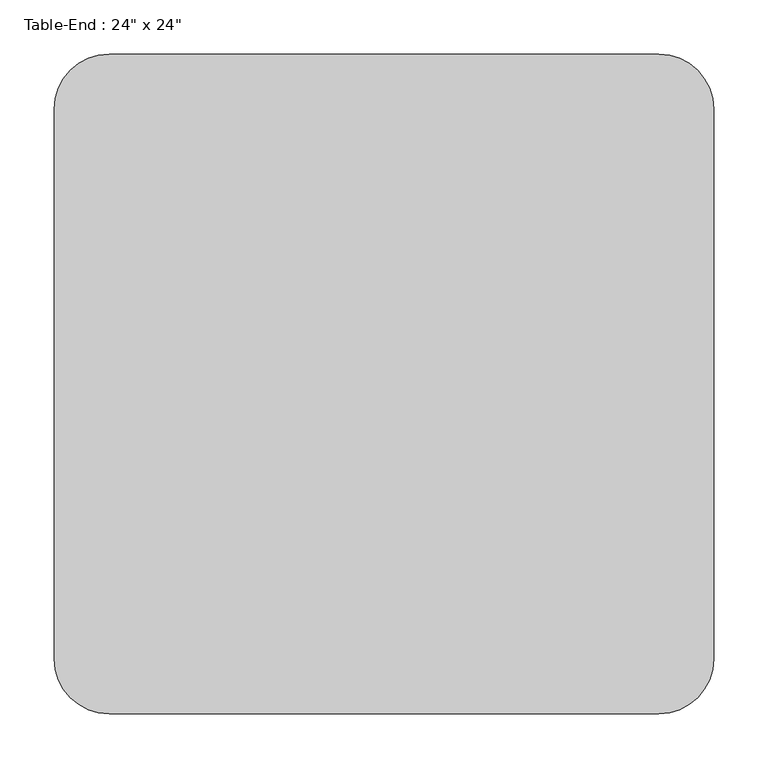
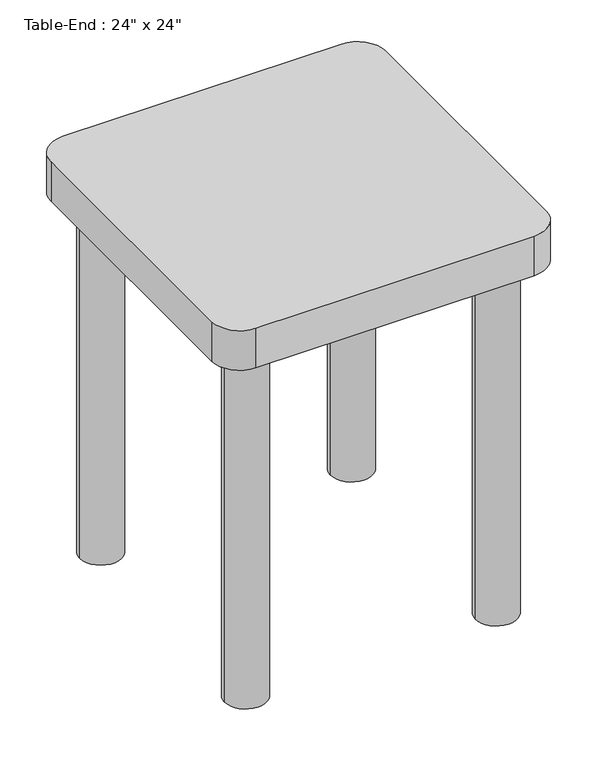
"""IFC4 building model written with IfcOpenShell, lengths in millimetres: furniture geometry."""

from ifc_helpers import new_model, si_unit, point, frame, frame_2d, origin, origin_with_axes, place, context, project, spatial, polyline, circle_curve, trimmed, segment, composite_curve, outline, extrude, source, transform, mapped, element, save


def furniture_bcf351fa(model_context):
    return source(origin(), model_context, "Body", "SweptSolid", [
        extrude(outline(composite_curve([segment(polyline([(562.5336303, -152.4), (54.5336303, -152.4)]), True, "CONTINUOUS"), segment(trimmed(circle_curve(frame_2d((54.5336303, -101.6)), 50.8), [point((54.5336303, -152.4))], [point((3.7336303, -101.6))], False, "CARTESIAN"), True, "CONTINUOUS"), segment(polyline([(3.7336303, -101.6), (3.7336303, 406.4)]), True, "CONTINUOUS"), segment(trimmed(circle_curve(frame_2d((54.5336303, 406.4)), 50.8), [point((3.7336303, 406.4))], [point((54.5336303, 457.2))], False, "CARTESIAN"), True, "CONTINUOUS"), segment(polyline([(54.5336303, 457.2), (562.5336303, 457.2)]), True, "CONTINUOUS"), segment(trimmed(circle_curve(frame_2d((562.5336303, 406.4)), 50.8), [point((562.5336303, 457.2))], [point((613.3336303, 406.4))], False, "CARTESIAN"), True, "CONTINUOUS"), segment(polyline([(613.3336303, 406.4), (613.3336303, -101.6)]), True, "CONTINUOUS"), segment(trimmed(circle_curve(frame_2d((562.5336303, -101.6)), 50.8), [point((613.3336303, -101.6))], [point((562.5336303, -152.4))], False, "CARTESIAN"), True, "CONTINUOUS")], self_intersect=False)), frame((0.0, 0.0, 685.8), z_axis=(0.0, 0.0, 1.0), x_axis=(1.0, 0.0, 0.0)), (0.0, 0.0, 1.0), 76.2),
        extrude(outline(composite_curve([segment(trimmed(circle_curve(frame_2d((79.9336303, 381.0)), 38.1), [point((41.8336303, 381.0))], [point((118.0336303, 381.0))], False, "CARTESIAN"), True, "CONTINUOUS"), segment(trimmed(circle_curve(frame_2d((79.9336303, 381.0)), 38.1), [point((118.0336303, 381.0))], [point((41.8336303, 381.0))], False, "CARTESIAN"), True, "CONTINUOUS")], self_intersect=False)), origin_with_axes(), (0.0, 0.0, 1.0), 685.8),
        extrude(outline(composite_curve([segment(trimmed(circle_curve(frame_2d((79.9336303, -76.2)), 38.1), [point((41.8336303, -76.2))], [point((118.0336303, -76.2))], False, "CARTESIAN"), True, "CONTINUOUS"), segment(trimmed(circle_curve(frame_2d((79.9336303, -76.2)), 38.1), [point((118.0336303, -76.2))], [point((41.8336303, -76.2))], False, "CARTESIAN"), True, "CONTINUOUS")], self_intersect=False)), origin_with_axes(), (0.0, 0.0, 1.0), 685.8),
        extrude(outline(composite_curve([segment(trimmed(circle_curve(frame_2d((537.1336303, -76.2)), 38.1), [point((499.0336303, -76.2))], [point((575.2336303, -76.2))], False, "CARTESIAN"), True, "CONTINUOUS"), segment(trimmed(circle_curve(frame_2d((537.1336303, -76.2)), 38.1), [point((575.2336303, -76.2))], [point((499.0336303, -76.2))], False, "CARTESIAN"), True, "CONTINUOUS")], self_intersect=False)), origin_with_axes(), (0.0, 0.0, 1.0), 685.8),
        extrude(outline(composite_curve([segment(trimmed(circle_curve(frame_2d((537.1336303, 381.0)), 38.1), [point((499.0336303, 381.0))], [point((575.2336303, 381.0))], False, "CARTESIAN"), True, "CONTINUOUS"), segment(trimmed(circle_curve(frame_2d((537.1336303, 381.0)), 38.1), [point((575.2336303, 381.0))], [point((499.0336303, 381.0))], False, "CARTESIAN"), True, "CONTINUOUS")], self_intersect=False)), origin_with_axes(), (0.0, 0.0, 1.0), 685.8),
    ])


if __name__ == "__main__":
    model = new_model("IFC4")
    model_context = context("Model", 3, world=origin())
    ifc_project = project(units=[si_unit("LENGTHUNIT", "METRE", prefix="MILLI")], contexts=[model_context])
    site = spatial("IfcSite", under=ifc_project)
    building = spatial("IfcBuilding", under=site)
    placement = place(None, origin())
    furniture_shape = furniture_bcf351fa(model_context)
    element("IfcFurniture", 1, ObjectType="Table-End : 24\" x 24\"", at=placement, inside=building, context=model_context, shape_type="MappedRepresentation", body=[
        mapped(furniture_shape, transform((0.0, 0.0, 0.0), x_axis=(1.0, 0.0, 0.0), y_axis=(0.0, 1.0, 0.0), z_axis=(0.0, 0.0, 1.0))),
    ])
    save(model, "model.ifc")

# Revit data of these elements
# Type "Table-End : 24\" x 24\""
#   Assembly Code = "E2020200"
#   Height = 2' - 6"
#   Length = 2' - 0"
#   Width = 2' - 0"
#   Base Material = Birch
#   Top Material = Laminate, Ivory, Matte
#   Default Elevation = 0
# Element 1 (IfcFurniture, "Table-End : 24\" x 24\"")
#   Materials on its faces: "Laminate, Ivory, Matte", "Birch"
# Materials
#   "Birch": class "Wood", colour RGB 224 178 126, transparency 0, Description = "Betula Alleghaniensis", Cost = 0
#   "Laminate, Ivory, Matte": class "Plastic", colour RGB 247 247 239, transparency 0, Description = "Plastic Laminate - Ivory, Matte", Cost = 0
